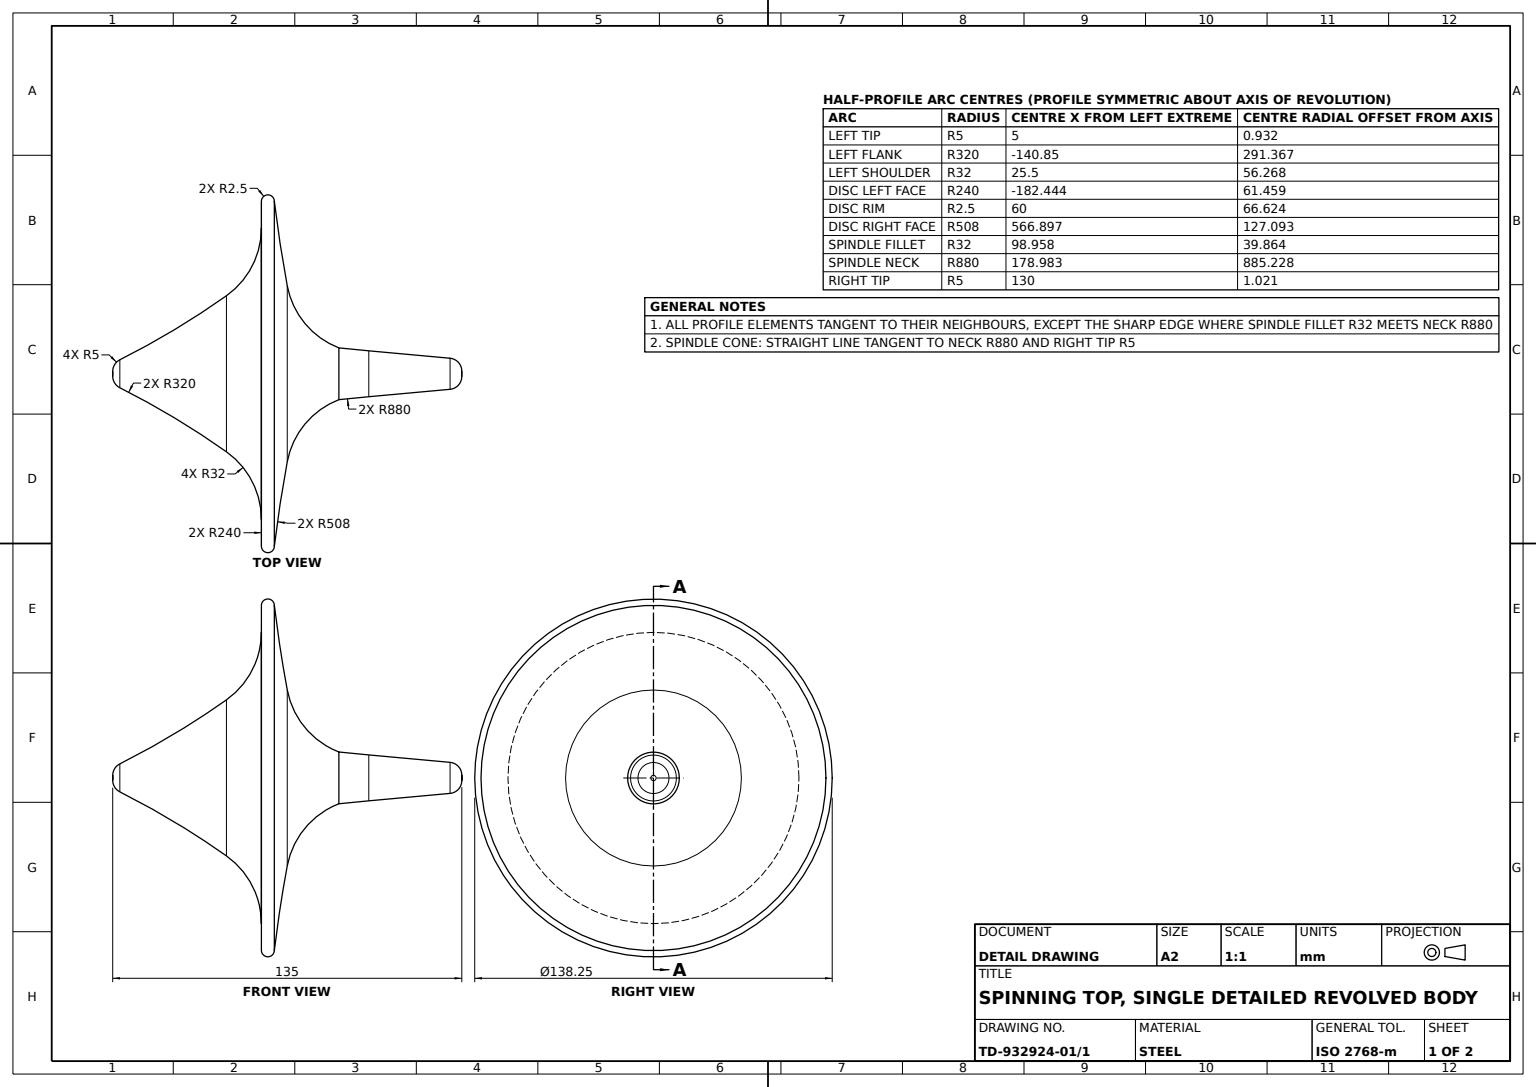
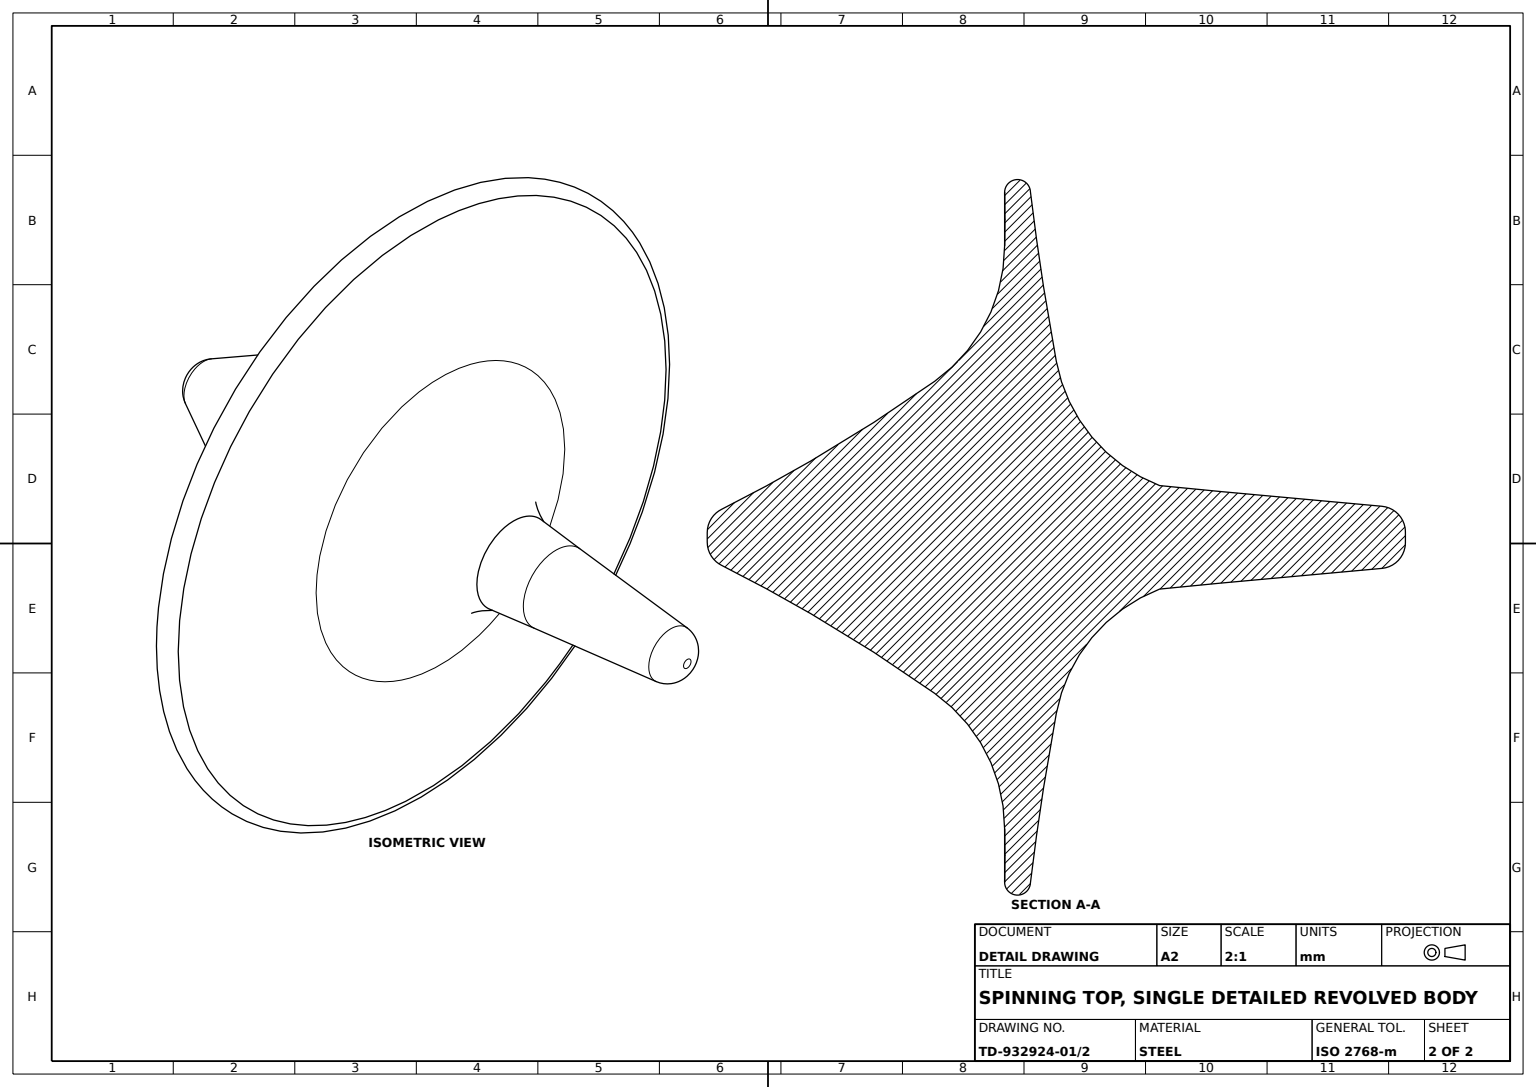
SolidWorks part; units mm, degrees
material "Plain Carbon Steel"
ref_plane "Front Plane" through (0, 0, 0) normal (0, 0, 1) x (1, 0, 0)
ref_plane "Top Plane" through (0, 0, 0) normal (0, 1, 0) x (1, 0, 0)
ref_plane "Right Plane" through (0, 0, 0) normal (1, 0, 0) x (0, 0, -1)
sketch "Top Half Profile" plane through (0, 0, 0) normal (0, 0, 1) x (1, 0, 0)
  line L0 (0, 67.5) -> (0, -67.5)
  line L1 (0, -67.5) -> (0.9318, -67.5)
  line L2 (6, 62.9631) -> (8.8674, 31.5329)
  line L3 (0, 67.5) -> (1.0215, 67.5)
  line L4 (34, 0) -> (34, -5) construction
  line L5 (17.7, -42.5) -> (0, -42.5) construction
  line L6 (0, 0) -> (34, 0) construction
  line L8 (34, -5) -> (34, -15) construction
  line L9 (34, -5) -> (66.6999, -5) construction
  line L10 (34, -15) -> (39.0924, -15) construction
  line L11 (34, -5) -> (34, -10) construction
  line L12 (34, -10) -> (66.6509, -10) construction
  arc A0 (6, 62.9631) -> (1.0215, 67.5) centre (1.0215, 62.5) ccw
  arc A1 (5.4, -64.7438) -> (0.9318, -67.5) centre (0.9318, -62.5) cw
  arc A2 (56.268, -10) -> (66.5708, -9.9983) centre (61.4594, -249.9438) cw
  arc A3 (8.8674, 31.5329) -> (10, 19.9631) centre (885.228, 111.4834) ccw
  arc A4 (10, 19.9631) -> (8.8674, 31.5329) centre (885.228, 111.4834) cw
  arc A5 (30.1459, -23.5166) -> (5.4, -64.7438) centre (291.3672, -208.3502) ccw
  arc A6 (34, 0) -> (10, 19.9631) centre (39.8641, 31.4581) cw
  arc A7 (66.6999, -5) -> (34, 0) centre (127.0928, 499.3974) cw
  arc A8 (30.1459, -23.5166) -> (56.268, -10) centre (56.268, -42) cw
  arc A9 (66.6999, -5) -> (66.5708, -9.9983) centre (66.624, -7.4988) cw
  dimension "D2" = 5
  dimension "D5" = 43
  dimension "D6" = 5
  dimension "D10" = 240
  dimension "D11" = 880
  dimension "D12" = 320
  dimension "D7" = 32
  dimension "D13" = 34
  dimension "D14" = 508
  dimension "D15" = 5
  dimension "D16" = 5.4
  dimension "D18" = 0
  dimension "D17" = 32
  dimension "D20" = 2.5
  dimension "D1" = 135
  dimension "D3" = 6
  dimension "D4" = 10
  dimension "D8" = 17.7
  dimension "D9" = 25
  dimension "D19" = 5
  dimension "D21" = 66.624
  dimension "D22" = 111.4834
  dimension "D23" = 66.6509
revolve "Spinning Top Revolve" add sketch "Top Half Profile" angle 360 about L0
